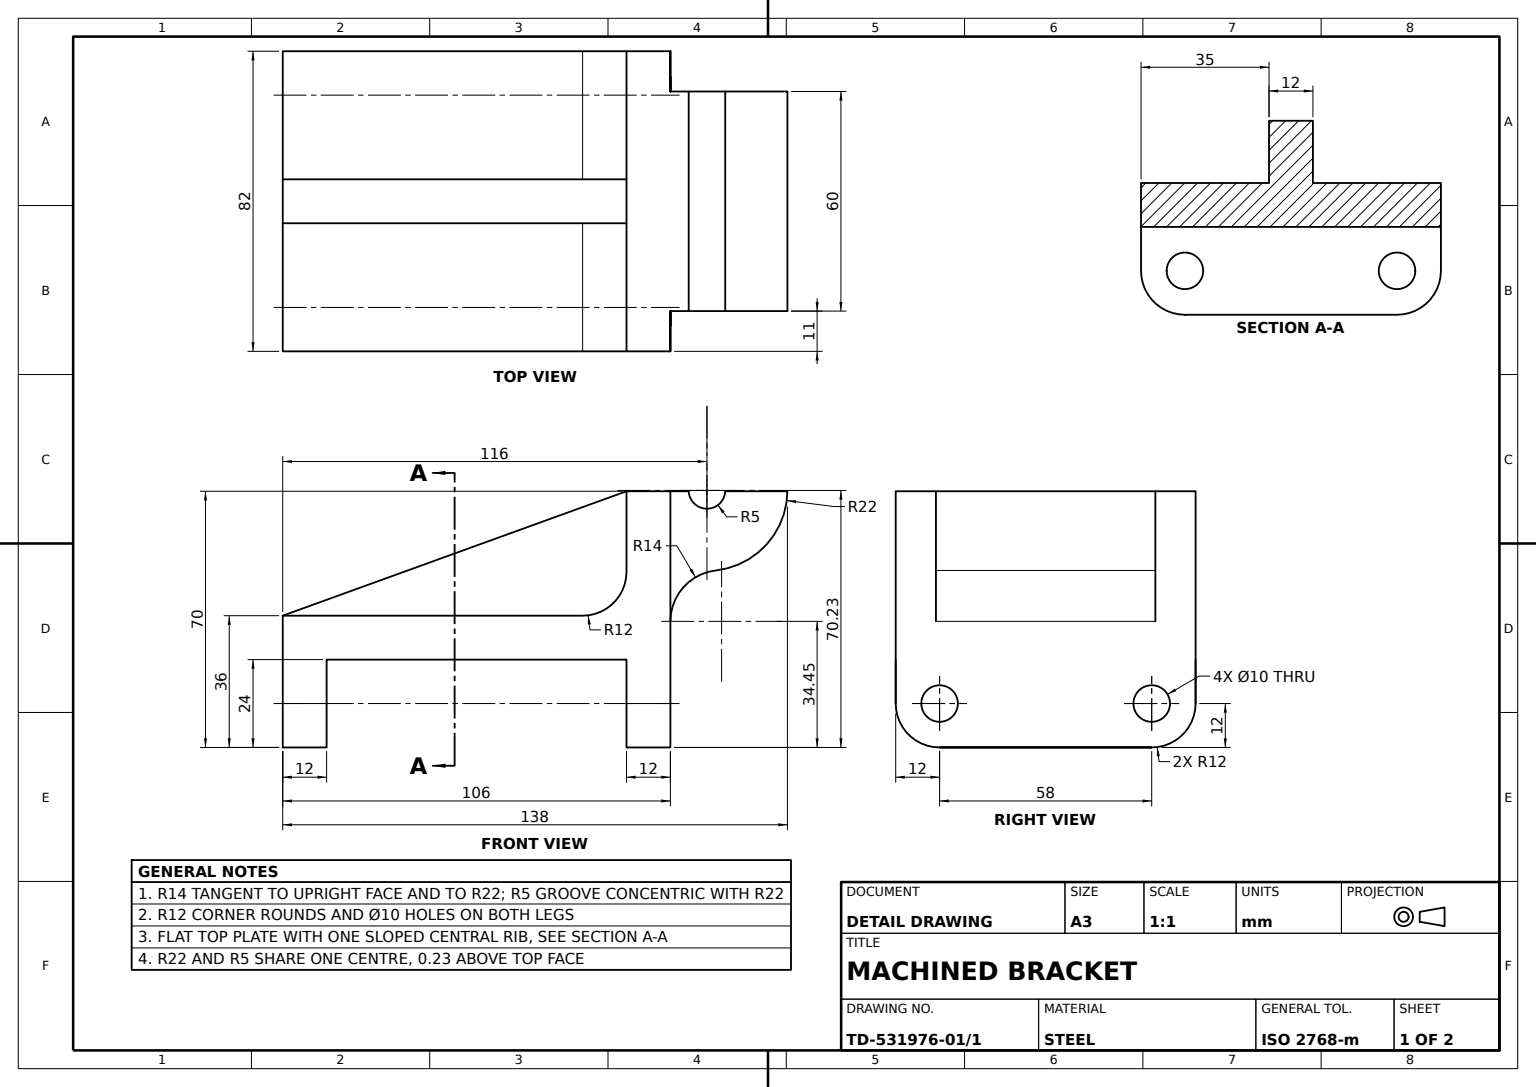
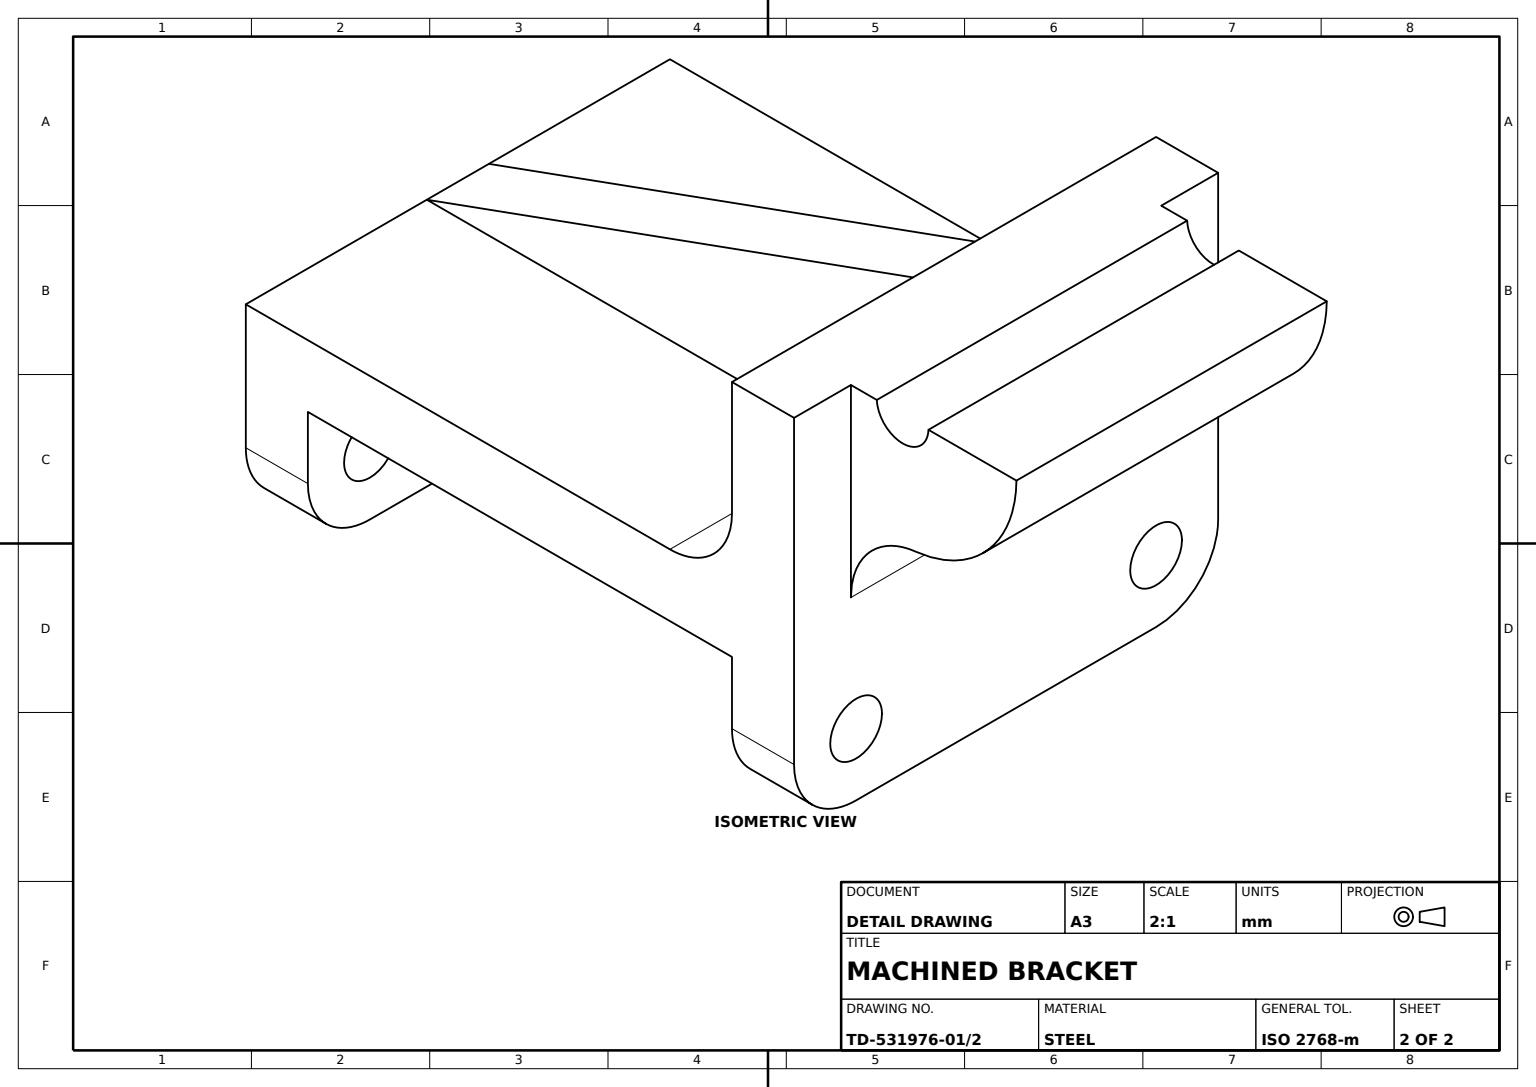
from build123d import *

# Parameters (mm, degrees)
BRACKET_BODY_DEPTH        = 82
BODY_CORNER_FILLETS_R12_R = 12
MOUNTING_HOLES_SKETCH_R   = 5
MOUNTING_HOLES_DEPTH      = 152.19523802
CENTRE_RIB_12MM_REACH     = 135.48
RIB_SKETCH_WALL_W         = 368.920663258
RIB_SKETCH_WALL_H         = 12
INNER_CORNER_FILLET_R12_R = 12
CRADLE_BOSS_DEPTH         = 30


with BuildPart() as part:
    # Bracket Profile Sketch → Bracket Body (new body)
    with BuildSketch(Plane(origin=(0, 0, 0), x_dir=(0, 0, -1), z_dir=(1, 0, 0))):
        Polygon((0, 0), (12, 0), (12, 24), (94, 24), (94, 0), (106, 0), (106, 70), (94, 70), (94, 36), (0, 36), align=None)
    extrude(amount=BRACKET_BODY_DEPTH)

    # Body Corner Fillets R12
    body_corner_fillets_r12_edges = [part.edges().sort_by_distance(p)[0] for p in [
        (0, 0, -100),
        (0, 0, -6),
        (82, 0, -100),
        (82, 0, -6),
    ]]
    fillet(body_corner_fillets_r12_edges, radius=BODY_CORNER_FILLETS_R12_R)

    # Mounting Holes Sketch → Mounting Holes (cut, through all)
    with BuildSketch(Plane.XY):
        with Locations((12, 12)):
            Circle(MOUNTING_HOLES_SKETCH_R)
        with Locations((70, 12)):
            Circle(MOUNTING_HOLES_SKETCH_R)
    extrude(amount=-MOUNTING_HOLES_DEPTH, mode=Mode.SUBTRACT)

    # Rib Sketch wall → Centre Rib 12mm (add, up to next)
    with BuildSketch(Plane(origin=(41, 53, -47), x_dir=(0, -0.340136081654, 0.940376225751), z_dir=(0, -0.940376225751, -0.340136081654)), mode=Mode.PRIVATE) as centre_rib_12mm_sk1:
        Rectangle(RIB_SKETCH_WALL_W, RIB_SKETCH_WALL_H)
    centre_rib_12mm_tool1 = extrude(centre_rib_12mm_sk1.sketch, amount=CENTRE_RIB_12MM_REACH, mode=Mode.PRIVATE) - part.part
    add(centre_rib_12mm_tool1.solids().sort_by_distance((41, 53, -47))[0])

    # Inner Corner Fillet R12
    inner_corner_fillet_r12_edges = [part.edges().sort_by_distance(p)[0] for p in [
        (64.5, 36, -94),
        (17.5, 36, -94),
    ]]
    fillet(inner_corner_fillet_r12_edges, radius=INNER_CORNER_FILLET_R12_R)

    # Cradle Profile Sketch → Cradle Boss (add, symmetric)
    with BuildSketch(Plane(origin=(41, 0, 0), x_dir=(0, 0, -1), z_dir=(1, 0, 0))):
        with BuildLine():
            Line((120.994884686, 70), (137.998837993, 70))
            ThreePointArc((137.998837993, 70), (132.322243398, 55.475371387), (118.444444444, 48.362336959))
            ThreePointArc((118.444444444, 48.362336959), (109.565016105, 43.782358433), (106, 34.449025099))
            Line((106, 34.449025099), (106, 70))
            Line((106, 70), (111.005115314, 70))
            ThreePointArc((111.005115314, 70), (116, 65.226112739), (120.994884686, 70))
        make_face()
    extrude(amount=CRADLE_BOSS_DEPTH, both=True)


solid = part.part
